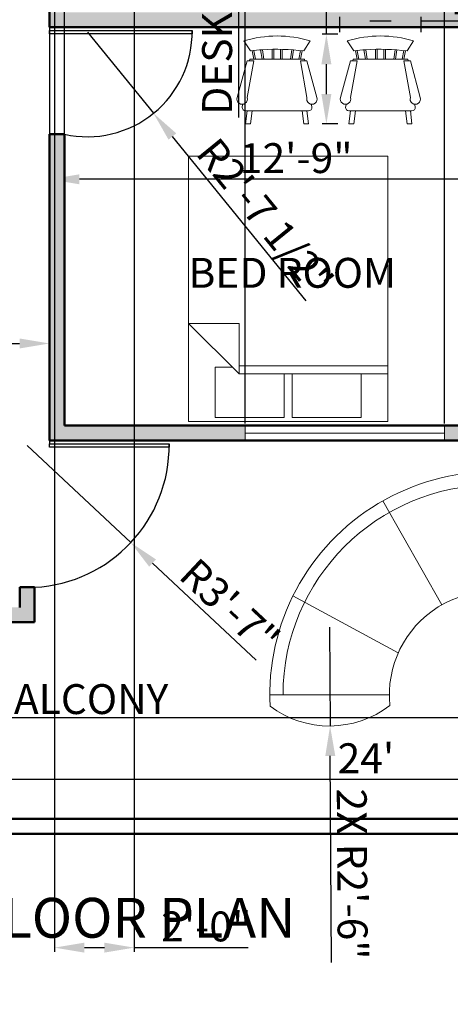
# Model space of a CAD drawing. Units: inches. Extents: x 875413 to 876020, y 447446 to 448210.
# Tile 3 of 8: x 875681 to 875810, y 447498 to 447795. Entities that reach past the tile are written whole.
import ezdxf

# ---------------------------------------------------------------- set-up
doc = ezdxf.new("R2010")
doc.units = ezdxf.units.IN
for name, color, linetype, lineweight in [('A-ANNO-DIMS', 2, 'Continuous', 13), ('A-ANNO-TEXT', 7, 'Continuous', 35), ('A-AREA-IDEN', 7, 'Continuous', 25), ('A-DOOR', 3, 'Continuous', 25), ('A-FURN', 8, 'Continuous', 18), ('A-GLAZ', 4, 'Continuous', 20), ('A-WALL', 7, 'Continuous', 50)]:
    doc.layers.add(name, color=color, linetype=linetype, lineweight=lineweight)
doc.layers.add('A-WALL-PATT', color=18, linetype='Continuous', lineweight=13, true_color=0x000000)
doc.styles.get("Standard").update_dxf_attribs({"font": 'arial.ttf'})
doc.dimstyles.new('ISO-25', dxfattribs={"dimtxt": 9, "dimasz": 9, "dimexe": 1.25, "dimexo": 0.625, "dimtad": 1, "dimdec": 1, "dimrnd": 9, "dimlunit": 3, "dimtxsty": 'Standard', "dimcen": 2.5, "dimadec": 0, "dimazin": 0, "dimtfac": 1, "dimtdec": 1, "dimtmove": 0, "dimatfit": 3, "dimfxl": 1, "dimarcsym": 0})

# ---------------------------------------------------------------- blocks, each defined once
blk = doc.blocks.new('*D19')
at = {"layer": 'A-ANNO-DIMS', "color": 0, "lineweight": -2, "transparency": 16777216}
for p, q in [((875643.2, 447554.64), (875643.2, 447567.26)), ((875652.2, 447566.01), (875917.7, 447566.01)), ((875926.7, 447554.64), (875926.7, 447567.26))]:
    blk.add_line(p, q, dxfattribs=at)
at = {"layer": 'A-ANNO-DIMS', "color": 0, "transparency": 16777216}
for points in [[(875652.2, 447567.51), (875652.2, 447564.51), (875643.2, 447566.01)], [(875917.7, 447567.51), (875917.7, 447564.51), (875926.7, 447566.01)]]:
    blk.add_solid(points, dxfattribs=at)
at = {"layer": 'Defpoints', "color": 0, "transparency": 16777216}
for p in [(875926.7, 447566.01), (875643.2, 447554.02), (875926.7, 447554.02)]:
    blk.add_point(p, dxfattribs=at)
at = {"layer": 'A-ANNO-DIMS', "color": 0, "transparency": 16777216, "insert": (875784.95, 447571.15), "char_height": 9, "attachment_point": 5}
blk.add_mtext("24'", dxfattribs=at)
blk = doc.blocks.new('*D24')
at = {"layer": 'A-ANNO-DIMS', "color": 0, "lineweight": -2, "transparency": 16777216}
for p, q in [((875689.7, 447791.89), (875689.7, 447745.44)), ((875838.2, 447791.89), (875838.2, 447745.44)), ((875829.2, 447746.69), (875698.7, 447746.69))]:
    blk.add_line(p, q, dxfattribs=at)
at = {"layer": 'A-ANNO-DIMS', "color": 0, "transparency": 16777216}
for points in [[(875698.7, 447748.19), (875698.7, 447745.19), (875689.7, 447746.69)], [(875829.2, 447748.19), (875829.2, 447745.19), (875838.2, 447746.69)]]:
    blk.add_solid(points, dxfattribs=at)
at = {"layer": 'Defpoints', "color": 0, "transparency": 16777216}
for p in [(875689.7, 447792.52), (875838.2, 447792.52), (875689.7, 447746.69)]:
    blk.add_point(p, dxfattribs=at)
at = {"layer": 'A-ANNO-DIMS', "color": 0, "transparency": 16777216, "insert": (875763.95, 447751.91), "char_height": 9, "attachment_point": 5}
blk.add_mtext('12\'-9"', dxfattribs=at)
blk = doc.blocks.new('Bed - Queen')
for p, q in [((0, -80.00003), (0, 0)), ((0, 0), (59.99999, 0)), ((59.99999, 0), (59.99999, -80.00003)), ((7.99999, -1.2), (28.79998, -1.2)), ((7.99999, -14.4), (7.99999, -1.2)), ((28.79998, -1.2), (28.79998, -14.4)), ((31.19999, -1.2), (51.99999, -1.2)), ((31.19999, -14.4), (31.19999, -1.2)), ((51.99999, -1.2), (51.99999, -16.4)), ((0, -14.4), (44.8, -14.4)), ((59.99999, -29.6), (44.8, -14.4)), ((44.8, -14.4), (44.8, -29.6)), ((44.8, -16.8), (0, -16.8)), ((51.99999, -16.4), (46.79936, -16.4)), ((44.8, -29.6), (59.99999, -29.6)), ((59.99999, -80.00003), (0, -80.00003))]:
    blk.add_line(p, q)
blk = doc.blocks.new('Chair - Rocking')
for p, q in [((-8, -4.5), (-10, -1.5)), ((8, -4.5), (10, -1.5)), ((-7.5, -4.5), (-7, -7)), ((-6.5, -7), (-7.02225, -4.43)), ((-4.5, -7), (-4.96674, -4.19951)), ((-4, -7), (-4.40532, -4.16272)), ((-1.5, -4.05012), (-1.5, -7)), ((-1, -7), (-1, -4.05012)), ((1, -7), (1, -4.04655)), ((1.5, -4.05012), (1.5, -7)), ((4, -7), (4.40187, -4.18694)), ((4.5, -7), (4.96761, -4.19437)), ((6.5, -7), (7, -4.4057)), ((7.5, -4.5), (7, -7)), ((-9, -7.5), (-12, -18.49999)), ((-7, -7.5), (-9, -7.5)), ((-9, -18.49999), (-7, -7.5)), ((-8.23428, -6.99939), (-8.3093, -7.47958)), ((-8.23041, -7), (8.23915, -7)), ((7, -7.5), (9, -7.5)), ((9, -18.49999), (7, -7.5)), ((8.31071, -7.48854), (8.23449, -7.00073)), ((9, -7.5), (12, -18.49999)), ((-10.36644, -20.64523), (-10.5, -21.49999)), ((10.5, -21.49999), (10.3575, -20.58798)), ((-9, -22.49999), (-9.5, -26.49999)), ((0, -22.49999), (-9.5, -22.49999)), ((-8, -26.49999), (-7.5, -22.49999)), ((0, -22.49999), (9.5, -22.49999)), ((8, -26.49999), (7.5, -22.49999)), ((9, -22.49999), (9.5, -26.49999)), ((-9.5, -26.49999), (-8, -26.49999)), ((9.5, -26.49999), (8, -26.49999))]:
    blk.add_line(p, q)
for centre, radius, start, end in [((0, -34.08333), 34.08333, 72.93847, 107.0615), ((0, -68.25004), 64.25, 93.92211, 97.15267), ((0, -68.25004), 64.25, 82.84733, 93.92211), ((-10.5, -18.99999), 1.58114, 161.5651, 18.43495), ((10.5, -18.99999), 1.58114, 161.5651, 18.43495), ((-9.5, -21.49999), 1, 180, 270), ((9.5, -21.49999), 1, 270, 0)]:
    blk.add_arc(centre, radius, start, end)
blk = doc.blocks.new('*D36')
at = {"layer": 'A-ANNO-DIMS', "color": 0, "lineweight": -2, "transparency": 16777216}
for p, q in [((875619.2, 447691.1), (875619.2, 447698.49)), ((875628.2, 447697.24), (875680.7, 447697.24)), ((875689.7, 447691.1), (875689.7, 447698.49))]:
    blk.add_line(p, q, dxfattribs=at)
at = {"layer": 'A-ANNO-DIMS', "color": 0, "transparency": 16777216}
for points in [[(875628.2, 447698.74), (875628.2, 447695.74), (875619.2, 447697.24)], [(875680.7, 447698.74), (875680.7, 447695.74), (875689.7, 447697.24)]]:
    blk.add_solid(points, dxfattribs=at)
at = {"layer": 'Defpoints', "color": 0, "transparency": 16777216}
for p in [(875689.7, 447697.24), (875619.2, 447690.48), (875689.7, 447690.48)]:
    blk.add_point(p, dxfattribs=at)
at = {"layer": 'A-ANNO-DIMS', "color": 0, "transparency": 16777216, "insert": (875654.45, 447702.46), "char_height": 9, "attachment_point": 5}
blk.add_mtext("6'", dxfattribs=at)
blk = doc.blocks.new('*D57')
at = {"layer": 'A-ANNO-DIMS', "color": 0, "lineweight": -2, "transparency": 16777216}
for p, q in [((875773.04, 447790.36), (875773.04, 447897.98)), ((875776.46, 447790.36), (875771.79, 447790.36)), ((875773.04, 447772.36), (875773.04, 447781.36)), ((875776.46, 447763.36), (875771.79, 447763.36))]:
    blk.add_line(p, q, dxfattribs=at)
at = {"layer": 'A-ANNO-DIMS', "color": 0, "transparency": 16777216}
for points in [[(875771.54, 447781.36), (875774.54, 447781.36), (875773.04, 447790.36)], [(875771.54, 447772.36), (875774.54, 447772.36), (875773.04, 447763.36)]]:
    blk.add_solid(points, dxfattribs=at)
at = {"layer": 'Defpoints', "color": 0, "transparency": 16777216}
for p in [(875773.04, 447790.36), (875777.09, 447790.36), (875777.09, 447763.36)]:
    blk.add_point(p, dxfattribs=at)
at = {"layer": 'A-ANNO-DIMS', "color": 0, "transparency": 16777216, "insert": (875767.76, 447848.67), "char_height": 9, "attachment_point": 5, "rotation": 90}
blk.add_mtext('CHAIR 2\'-3" TYP.', dxfattribs=at)
blk = doc.blocks.new('*D58')
at = {"layer": 'A-ANNO-DIMS', "color": 0, "lineweight": -2, "transparency": 16777216}
for p, q in [((875777.09, 447790.98), (875777.09, 447795.66)), ((875786.09, 447794.41), (875792.52, 447794.41)), ((875801.52, 447790.98), (875801.52, 447795.66)), ((875801.52, 447794.41), (875887.76, 447794.41))]:
    blk.add_line(p, q, dxfattribs=at)
at = {"layer": 'A-ANNO-DIMS', "color": 0, "transparency": 16777216}
for points in [[(875786.09, 447795.91), (875786.09, 447792.91), (875777.09, 447794.41)], [(875792.52, 447795.91), (875792.52, 447792.91), (875801.52, 447794.41)]]:
    blk.add_solid(points, dxfattribs=at)
at = {"layer": 'Defpoints', "color": 0, "transparency": 16777216}
for p in [(875801.52, 447794.41), (875777.09, 447790.36), (875801.52, 447790.36)]:
    blk.add_point(p, dxfattribs=at)
at = {"layer": 'A-ANNO-DIMS', "color": 0, "transparency": 16777216, "insert": (875849.14, 447799.69), "char_height": 9, "attachment_point": 5}
blk.add_mtext('2\'-0 1/2" TYP.', dxfattribs=at)
blk = doc.blocks.new('*D61')
at = {"layer": 'A-ANNO-DIMS', "color": 0, "lineweight": -2, "transparency": 16777216}
for p, q in [((875754.96, 447896.77), (875745.33, 447896.77)), ((875746.58, 447887.77), (875746.58, 447845.77)), ((875754.96, 447836.77), (875745.33, 447836.77)), ((875746.58, 447836.77), (875746.58, 447765.31))]:
    blk.add_line(p, q, dxfattribs=at)
at = {"layer": 'A-ANNO-DIMS', "color": 0, "transparency": 16777216}
for points in [[(875745.08, 447887.77), (875748.08, 447887.77), (875746.58, 447896.77)], [(875745.08, 447845.77), (875748.08, 447845.77), (875746.58, 447836.77)]]:
    blk.add_solid(points, dxfattribs=at)
at = {"layer": 'Defpoints', "color": 0, "transparency": 16777216}
for p in [(875755.58, 447896.77), (875746.58, 447836.77), (875755.58, 447836.77)]:
    blk.add_point(p, dxfattribs=at)
at = {"layer": 'A-ANNO-DIMS', "color": 0, "transparency": 16777216, "insert": (875741.3, 447796.54), "char_height": 9, "attachment_point": 5, "rotation": 90}
blk.add_mtext('DESK 5\'-0"', dxfattribs=at)
blk = doc.blocks.new('*D79')
at = {"layer": 'A-ANNO-DIMS', "color": 0, "lineweight": -2, "transparency": 16777216}
for p, q in [((875694.2, 447673.14), (875694.2, 448110.02)), ((875703.2, 448108.77), (875739.63, 448108.77)), ((875748.63, 447673.14), (875748.63, 448110.02))]:
    blk.add_line(p, q, dxfattribs=at)
at = {"layer": 'A-ANNO-DIMS', "color": 0, "transparency": 16777216}
for points in [[(875703.2, 448110.27), (875703.2, 448107.27), (875694.2, 448108.77)], [(875739.63, 448110.27), (875739.63, 448107.27), (875748.63, 448108.77)]]:
    blk.add_solid(points, dxfattribs=at)
at = {"layer": 'Defpoints', "color": 0, "transparency": 16777216}
for p in [(875748.63, 448108.77), (875694.2, 447672.52), (875748.63, 447672.52)]:
    blk.add_point(p, dxfattribs=at)
at = {"layer": 'A-ANNO-DIMS', "color": 0, "transparency": 16777216, "insert": (875721.42, 448114.05), "char_height": 9, "attachment_point": 5}
blk.add_mtext('4\'-6 1/2"', dxfattribs=at)
blk = doc.blocks.new('*D80')
at = {"layer": 'A-ANNO-DIMS', "color": 0, "lineweight": -2, "transparency": 16777216}
for p, q in [((875748.63, 447673.14), (875748.63, 448110.02)), ((875757.63, 448108.77), (875799.63, 448108.77)), ((875808.63, 447673.14), (875808.63, 448110.02))]:
    blk.add_line(p, q, dxfattribs=at)
at = {"layer": 'A-ANNO-DIMS', "color": 0, "transparency": 16777216}
for points in [[(875757.63, 448110.27), (875757.63, 448107.27), (875748.63, 448108.77)], [(875799.63, 448110.27), (875799.63, 448107.27), (875808.63, 448108.77)]]:
    blk.add_solid(points, dxfattribs=at)
at = {"layer": 'Defpoints', "color": 0, "transparency": 16777216}
for p in [(875808.63, 448108.77), (875748.63, 447672.52), (875808.63, 447672.52)]:
    blk.add_point(p, dxfattribs=at)
at = {"layer": 'A-ANNO-DIMS', "color": 0, "transparency": 16777216, "insert": (875778.63, 448113.99), "char_height": 9, "attachment_point": 5}
blk.add_mtext('5\'-0"', dxfattribs=at)
blk = doc.blocks.new('*D83')
at = {"layer": 'A-ANNO-DIMS', "color": 0, "lineweight": -2, "transparency": 16777216}
for p, q in [((875497.15, 447584.59), (875966.7, 447584.59)), ((875965.45, 447575.59), (875965.45, 447563.02)), ((875471.33, 447554.02), (875966.7, 447554.02)), ((875965.45, 447554.02), (875965.45, 447498.72))]:
    blk.add_line(p, q, dxfattribs=at)
at = {"layer": 'A-ANNO-DIMS', "color": 0, "transparency": 16777216}
for points in [[(875963.95, 447575.59), (875966.95, 447575.59), (875965.45, 447584.59)], [(875963.95, 447563.02), (875966.95, 447563.02), (875965.45, 447554.02)]]:
    blk.add_solid(points, dxfattribs=at)
at = {"layer": 'Defpoints', "color": 0, "transparency": 16777216}
for p in [(875496.52, 447584.59), (875470.7, 447554.02), (875965.45, 447554.02)]:
    blk.add_point(p, dxfattribs=at)
at = {"layer": 'A-ANNO-DIMS', "color": 0, "transparency": 16777216, "insert": (875960.17, 447521.87), "char_height": 9, "attachment_point": 5, "rotation": 90}
blk.add_mtext('2\'-6 1/2"', dxfattribs=at)
blk = doc.blocks.new('*D86')
at = {"layer": 'A-ANNO-DIMS', "color": 0, "lineweight": -2, "transparency": 16777216}
for p, q in [((875691.2, 447925.39), (875691.2, 447514.02)), ((875715.2, 447925.39), (875715.2, 447514.02)), ((875700.2, 447515.27), (875706.2, 447515.27)), ((875715.2, 447515.27), (875749.53, 447515.27))]:
    blk.add_line(p, q, dxfattribs=at)
at = {"layer": 'A-ANNO-DIMS', "color": 0, "transparency": 16777216}
for points in [[(875700.2, 447516.77), (875700.2, 447513.77), (875691.2, 447515.27)], [(875706.2, 447516.77), (875706.2, 447513.77), (875715.2, 447515.27)]]:
    blk.add_solid(points, dxfattribs=at)
at = {"layer": 'Defpoints', "color": 0, "transparency": 16777216}
for p in [(875691.2, 447926.02), (875715.2, 447926.02), (875715.2, 447515.27)]:
    blk.add_point(p, dxfattribs=at)
at = {"layer": 'A-ANNO-DIMS', "color": 0, "transparency": 16777216, "insert": (875736.87, 447520.49), "char_height": 9, "attachment_point": 5}
blk.add_mtext('2\'-0"', dxfattribs=at)
blk = doc.blocks.new('*D91')
at = {"layer": 'A-ANNO-DIMS', "color": 0, "lineweight": -2, "transparency": 16777216}
for p, q in [((875773.97, 447611.83), (875774.15, 447582.03)), ((875774.59, 447510.75), (875774.21, 447573.03))]:
    blk.add_line(p, q, dxfattribs=at)
at = {"layer": 'A-ANNO-DIMS', "color": 0, "transparency": 16777216}
blk.add_solid([(875775.71, 447573.04), (875772.71, 447573.02), (875774.15, 447582.03)], dxfattribs=at)
at = {"layer": 'Defpoints', "color": 0, "transparency": 16777216}
for p in [(875773.97, 447611.83), (875774.15, 447582.03)]:
    blk.add_point(p, dxfattribs=at)
at = {"layer": 'A-ANNO-DIMS', "color": 0, "transparency": 16777216, "insert": (875779.65, 447537.42), "char_height": 9, "attachment_point": 5, "rotation": 270.3552}
blk.add_mtext('2X R2\'-6"', dxfattribs=at)
blk = doc.blocks.new('*D93')
at = {"layer": 'A-ANNO-DIMS', "color": 0, "lineweight": -2, "transparency": 16777216}
for p, q in [((875682.93, 447666.52), (875714.15, 447637.27)), ((875751.94, 447601.86), (875720.71, 447631.12))]:
    blk.add_line(p, q, dxfattribs=at)
at = {"layer": 'A-ANNO-DIMS', "color": 0, "transparency": 16777216}
blk.add_solid([(875721.74, 447632.21), (875719.69, 447630.02), (875714.15, 447637.27)], dxfattribs=at)
at = {"layer": 'Defpoints', "color": 0, "transparency": 16777216}
for p in [(875682.93, 447666.52), (875714.15, 447637.27)]:
    blk.add_point(p, dxfattribs=at)
at = {"layer": 'A-ANNO-DIMS', "color": 0, "transparency": 16777216, "insert": (875743.18, 447617.23), "char_height": 9, "attachment_point": 5, "rotation": 316.8664}
blk.add_mtext('R3\'-7"', dxfattribs=at)
blk = doc.blocks.new('*D97')
at = {"layer": 'A-ANNO-DIMS', "color": 0, "lineweight": -2, "transparency": 16777216}
for p, q in [((875701.12, 447791.02), (875721, 447766.57)), ((875766.9, 447710.12), (875726.68, 447759.59))]:
    blk.add_line(p, q, dxfattribs=at)
at = {"layer": 'A-ANNO-DIMS', "color": 0, "transparency": 16777216}
blk.add_solid([(875727.84, 447760.53), (875725.51, 447758.64), (875721, 447766.57)], dxfattribs=at)
at = {"layer": 'Defpoints', "color": 0, "transparency": 16777216}
for p in [(875701.12, 447791.02), (875721, 447766.57)]:
    blk.add_point(p, dxfattribs=at)
at = {"layer": 'A-ANNO-DIMS', "color": 0, "transparency": 16777216, "insert": (875753.72, 447734.69), "char_height": 9, "attachment_point": 5, "rotation": 309.1118}
blk.add_mtext('R2\'-7 1/2"', dxfattribs=at)

msp = doc.modelspace()

# ---------------------------------------------------------------- hatches: boundary and pattern name
at = {"layer": 'A-WALL-PATT'}
h = msp.add_hatch(color=256, dxfattribs=at)
h.dxf.hatch_style = 1
h.paths.add_polyline_path([(875470.7, 447985.13), (875461.7, 447985.13), (875461.7, 447865.29), (875470.7, 447865.29), (875470.7, 447881.02), (875566.7, 447881.02), (875566.7, 447797.02), (875571.2, 447797.02), (875571.2, 447885.52), (875571.2, 447921.52), (875603.29, 447921.52), (875603.29, 447926.02), (875501.27, 447926.02), (875501.27, 447921.52), (875566.7, 447921.52), (875566.7, 447885.52), (875470.7, 447885.52), (875470.7, 447921.52), (875470.7, 447926.02)])
h.paths.add_polyline_path([(875470.7, 448070.02), (875518.96, 448070.02), (875518.96, 448079.02), (875461.7, 448079.02), (875461.7, 448045.13), (875470.7, 448045.13)])
h.paths.add_polyline_path([(875819.9, 448079.02), (875578.96, 448079.02), (875578.96, 448070.02), (875638.7, 448070.02), (875638.7, 447921.52), (875643.2, 447921.52), (875643.2, 448070.02), (875763.2, 448070.02), (875763.2, 447921.52), (875767.7, 447921.52), (875767.7, 448070.02), (875819.9, 448070.02)])
h.paths.add_polyline_path([(875935.7, 447978.92), (875926.7, 447978.92), (875926.7, 447926.02), (875926.7, 447921.52), (875926.7, 447885.52), (875842.7, 447885.52), (875842.7, 447921.52), (875899.7, 447921.52), (875899.7, 447926.02), (875805.34, 447926.02), (875805.34, 447921.52), (875838.2, 447921.52), (875838.2, 447885.52), (875838.2, 447797.02), (875689.7, 447797.02), (875689.7, 447792.52), (875842.7, 447792.52), (875842.7, 447881.02), (875926.7, 447881.02), (875926.7, 447857.16), (875935.7, 447857.16)])
h.paths.add_polyline_path([(875935.7, 448079.02), (875879.9, 448079.02), (875879.9, 448070.02), (875926.7, 448070.02), (875926.7, 448038.92), (875935.7, 448038.92)])
h.paths.add_polyline_path([(875935.7, 447833.16), (875926.7, 447833.16), (875926.7, 447797.02), (875842.7, 447797.02), (875842.7, 447792.52), (875926.7, 447792.52), (875926.7, 447756.52), (875935.7, 447756.52)])
h.paths.add_polyline_path([(875935.7, 447732.52), (875926.7, 447732.52), (875926.7, 447692.75, -0.007222), (875926.81, 447692.41, -0.08192), (875927.45, 447687.6, -0.071798), (875926.7, 447683.4), (875926.7, 447672.52), (875808.63, 447672.52), (875808.63, 447668.02), (875926.7, 447668.02), (875926.7, 447663.19), (875935.7, 447663.19)])
h.paths.add_polyline_path([(875842.7, 447792.52), (875838.2, 447792.52), (875838.2, 447704.02), (875842.7, 447704.02)])
h.paths.add_polyline_path([(875470.7, 447792.52), (875619.2, 447792.52), (875619.2, 447797.02), (875470.7, 447797.02), (875470.7, 447841.29), (875461.7, 447841.29), (875461.7, 447764.71), (875470.7, 447764.71)])
h.paths.add_polyline_path([(875619.2, 447760.51), (875616.95, 447760.51, -0.018388), (875614.7, 447760.37), (875614.7, 447672.52), (875470.7, 447672.52), (875470.7, 447704.71), (875461.7, 447704.71), (875461.7, 447640.7), (875470.7, 447640.7), (875470.7, 447668.02), (875619.2, 447668.02)])
h.paths.add_polyline_path([(875511.12, 447554.02), (875470.7, 447554.02), (875470.7, 447580.7), (875461.7, 447580.7), (875461.7, 447545.02), (875511.12, 447545.02)])
h.paths.add_polyline_path([(875656.47, 447554.02), (875620.05, 447554.02, -0.057036), (875616.67, 447553.74, -0.040891), (875614.26, 447554.02), (875571.12, 447554.02), (875571.12, 447545.02), (875656.47, 447545.02)])
h.paths.add_polyline_path([(875643.2, 447613.27), (875685.21, 447613.27), (875685.21, 447617.77), (875685.21, 447623.8), (875680.71, 447623.8), (875680.71, 447617.77), (875618.23, 447617.77), (875618.23, 447623.8), (875613.73, 447623.8), (875613.73, 447617.77), (875613.73, 447613.27), (875638.7, 447613.27), (875638.7, 447554.02), (875643.2, 447554.02)])
h.paths.add_polyline_path([(875694.2, 447760.28), (875689.7, 447760.28), (875689.7, 447668.02), (875748.63, 447668.02), (875748.63, 447672.52), (875694.2, 447672.52)])

# ---------------------------------------------------------------- linework, layer by layer
at = {"layer": 'A-DOOR'}
for p, q in [((875689.7, 447792.52), (875689.7, 447791.52)), ((875689.7, 447791.52), (875725.7, 447791.52)), ((875689.7, 447790.52), (875689.7, 447791.52)), ((875725.7, 447791.52), (875732.63, 447791.52)), ((875732.63, 447791.52), (875732.63, 447790.52)), ((875732.63, 447790.52), (875689.7, 447790.52)), ((875689.7, 447668.02), (875689.7, 447667.02)), ((875689.7, 447667.02), (875725.7, 447667.02)), ((875689.7, 447666.02), (875689.7, 447667.02)), ((875725.7, 447667.02), (875725.7, 447666.02)), ((875725.7, 447666.02), (875689.7, 447666.02))]:
    msp.add_line(p, q, dxfattribs=at)
for centre, radius, start, end in [((875701.12, 447791.02), 31.51, 257.3126, 0.9093), ((875682.93, 447666.52), 42.78, 273.0621, 0.6697)]:
    msp.add_arc(centre, radius, start, end, dxfattribs=at)
at = {"layer": 'A-FURN'}
for p, q in [((875807.78, 447618.52), (875789.98, 447649.82)), ((875794.69, 447604.09), (875762.97, 447621.2)), ((875791.99, 447591.38), (875755.99, 447591.38))]:
    msp.add_line(p, q, dxfattribs=at)
for centre, radius, start, end in [((875823.22, 447591.38), 67.23, 357.2076, 182.8871), ((875823.22, 447591.38), 63.23, 0, 180), ((875823.22, 447591.38), 31.23, 354.002, 185.813), ((875773.97, 447611.83), 29.81, 233.1121, 307.5973)]:
    msp.add_arc(centre, radius, start, end, dxfattribs=at)
at = {"layer": 'A-GLAZ'}
for p, q in [((875748.63, 447672.52), (875748.63, 447668.02)), ((875808.63, 447672.52), (875808.63, 447668.02)), ((875748.63, 447670.27), (875808.63, 447670.27))]:
    msp.add_line(p, q, dxfattribs=at)
at = {"layer": 'A-WALL'}
for p, q in [((875689.7, 447792.52), (875689.7, 447797.02)), ((875926.7, 447792.52), (875689.7, 447792.52)), ((875689.7, 447668.02), (875689.7, 447760.28)), ((875689.7, 447760.28), (875694.2, 447760.28)), ((875694.2, 447672.52), (875694.2, 447760.28)), ((875926.7, 447672.52), (875694.2, 447672.52)), ((875926.7, 447668.02), (875689.7, 447668.02)), ((875680.71, 447617.77), (875680.71, 447623.8)), ((875680.71, 447623.8), (875685.21, 447623.8)), ((875685.21, 447623.8), (875685.21, 447617.77)), ((875685.21, 447613.27), (875685.21, 447617.77)), ((875643.2, 447613.27), (875685.21, 447613.27)), ((875656.47, 447554.02), (875926.7, 447554.02)), ((875656.47, 447549.52), (875931.2, 447549.52))]:
    msp.add_line(p, q, dxfattribs=at)

# ---------------------------------------------------------------- block references
at = {"layer": 'A-FURN'}
for p in [(875758.2, 447789.86), (875789.31, 447789.86)]:
    msp.add_blockref('Chair - Rocking', p, dxfattribs=at)
at = {"layer": 'A-FURN', "rotation": 180}
msp.add_blockref('Bed - Queen', (875791.55, 447673.71), dxfattribs=at)

# ---------------------------------------------------------------- texts
at = {"layer": 'A-ANNO-TEXT', "insert": (875618.96, 447530.26), "char_height": 12, "attachment_point": 1}
msp.add_mtext_dynamic_manual_height_columns('FIRST FLOOR PLAN', width=417.4622, gutter_width=12.5, heights=[0], dxfattribs=at)
at = {"layer": 'A-AREA-IDEN', "char_height": 9, "attachment_point": 1}
for s, insert in [('BED ROOM', (875731.55, 447723.02)), ('BALCONY', (875670.9, 447594.63))]:
    msp.add_mtext_dynamic_manual_height_columns(s, width=100.7812, gutter_width=12.5, heights=[0], dxfattribs=dict(at, insert=insert))

# ---------------------------------------------------------------- dimensions: what is measured, and where the dimension line sits
at = {"layer": 'A-ANNO-DIMS'}
for base, p1, p2, override, picture, middle in [((875748.63, 448108.77), (875694.2, 447672.52), (875748.63, 447672.52), {"dimdec": 1, "dimlfac": 1, "dimrnd": 0, "dimzin": 1, "dimdsep": 46, "dimlunit": 4, "dimfrac": 2}, '*D79', (875721.42, 448114.05)), ((875808.63, 448108.77), (875748.63, 447672.52), (875808.63, 447672.52), {"dimdec": 1, "dimlfac": 1, "dimrnd": 0, "dimzin": 1, "dimdsep": 46, "dimlunit": 4, "dimfrac": 2}, '*D80', (875778.63, 448113.99)), ((875715.2, 447515.27), (875691.2, 447926.02), (875715.2, 447926.02), {"dimdec": 1, "dimlfac": 1, "dimrnd": 0, "dimzin": 1, "dimdsep": 46, "dimlunit": 4, "dimfrac": 2}, '*D86', (875736.87, 447520.49)), ((875689.7, 447746.69), (875838.2, 447792.52), (875689.7, 447792.52), {"dimclrd": 0, "dimclre": 0, "dimclrt": 0}, '*D24', (875763.95, 447751.91)), ((875689.7, 447697.24), (875619.2, 447690.48), (875689.7, 447690.48), {"dimclrd": 0, "dimclre": 0, "dimclrt": 0}, '*D36', (875654.45, 447702.46)), ((875926.7, 447566.01), (875643.2, 447554.02), (875926.7, 447554.02), {"dimclrd": 0, "dimclre": 0, "dimclrt": 0}, '*D19', (875784.95, 447571.15))]:
    dim = msp.add_linear_dim(base=base, p1=p1, p2=p2, dimstyle='ISO-25', override=override, dxfattribs=at)
    dim.commit()
    dim.dimension.update_dxf_attribs({"geometry": picture, "text_midpoint": middle})
for base, p1, p2, angle, text, picture, middle in [((875773.04, 447790.36), (875777.09, 447763.36), (875777.09, 447790.36), 90, 'CHAIR <> TYP.', '*D57', (875767.76, 447848.67)), ((875746.58, 447836.77), (875755.58, 447896.77), (875755.58, 447836.77), 270, 'DESK <>', '*D61', (875741.3, 447796.54))]:
    dim = msp.add_linear_dim(base=base, p1=p1, p2=p2, angle=angle, text=text, dimstyle='ISO-25', override={"dimdec": 1, "dimlfac": 1, "dimrnd": 0, "dimzin": 1, "dimdsep": 46, "dimlunit": 4, "dimfrac": 2}, dxfattribs=at)
    dim.commit()
    dim.dimension.update_dxf_attribs({"geometry": picture, "text_midpoint": middle})
dim = msp.add_linear_dim(base=(875801.52, 447794.41), p1=(875777.09, 447790.36), p2=(875801.52, 447790.36), text='<> TYP.', dimstyle='ISO-25', override={"dimdec": 1, "dimlfac": 1, "dimrnd": 0, "dimzin": 1, "dimdsep": 46, "dimlunit": 4, "dimfrac": 2}, dxfattribs=at)
dim.commit()
dim.dimension.update_dxf_attribs({"geometry": '*D58', "text_midpoint": (875849.14, 447799.69)})
for center, mpoint, picture, middle in [((875701.12, 447791.02), (875721, 447766.57), '*D97', (875753.72, 447734.69)), ((875682.93, 447666.52), (875714.15, 447637.27), '*D93', (875743.18, 447617.23))]:
    dim = msp.add_radius_dim(center=center, mpoint=mpoint, dimstyle='ISO-25', override={"dimdec": 1, "dimlfac": 1, "dimrnd": 0, "dimzin": 1, "dimdsep": 46, "dimlunit": 4, "dimfrac": 2}, dxfattribs=at)
    dim.commit()
    dim.dimension.update_dxf_attribs({"geometry": picture, "text_midpoint": middle})
dim = msp.add_radius_dim(center=(875773.97, 447611.83), mpoint=(875774.15, 447582.03), text='2X <>', dimstyle='ISO-25', override={"dimdec": 1, "dimlfac": 1, "dimrnd": 0, "dimzin": 1, "dimdsep": 46, "dimlunit": 4, "dimfrac": 2}, dxfattribs=at)
dim.commit()
dim.dimension.update_dxf_attribs({"geometry": '*D91', "text_midpoint": (875779.65, 447537.42)})
dim = msp.add_linear_dim(base=(875965.45, 447554.02), p1=(875496.52, 447584.59), p2=(875470.7, 447554.02), angle=90, dimstyle='ISO-25', override={"dimdec": 1, "dimlfac": 1, "dimrnd": 0, "dimzin": 1, "dimdsep": 46, "dimlunit": 4, "dimfrac": 2}, dxfattribs=at)
dim.commit()
dim.dimension.update_dxf_attribs({"geometry": '*D83', "text_midpoint": (875960.17, 447521.87)})

doc.saveas('drawing.dxf')
